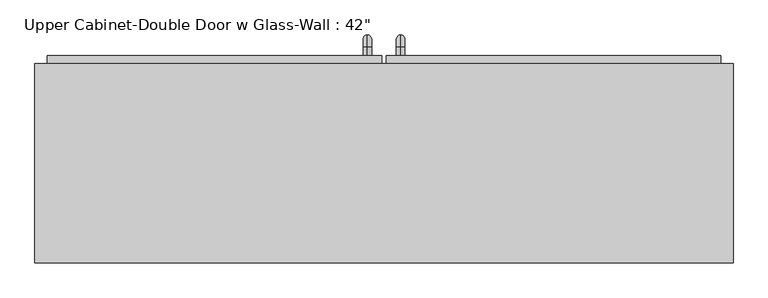
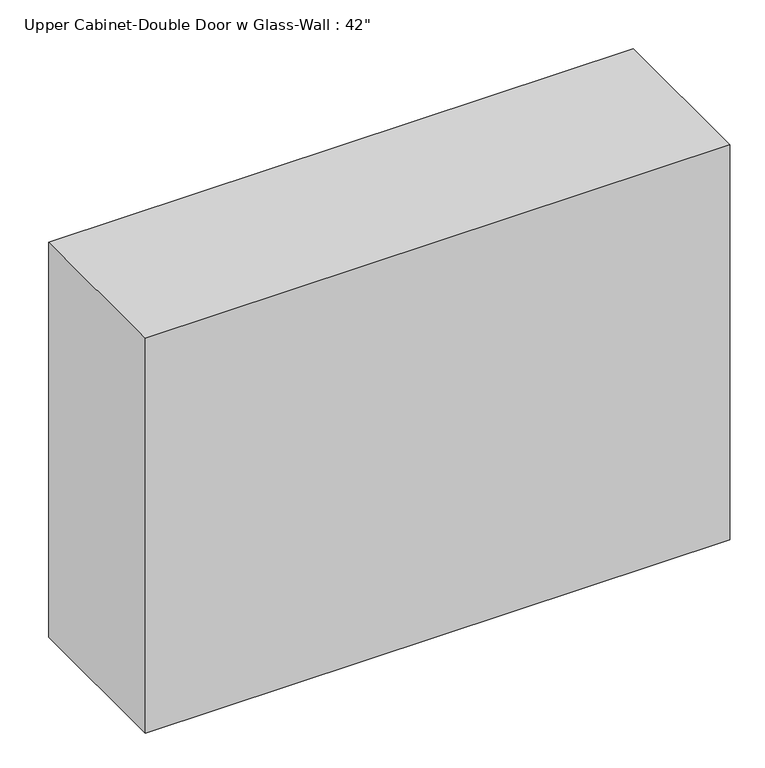
"""IFC4 building model written with IfcOpenShell, lengths in millimetres: furniture geometry."""

from ifc_helpers import new_model, si_unit, point, frame, origin, place, context, project, spatial, polyline, circle_curve, ellipse_curve, trimmed, outline, extrude, faceted_brep, source, transform, mapped, element, save
from ifc_brep_helpers import plane_surface, cylinder_surface, revolved_surface, advanced_brep


def furniture_19fd8281(model_context):
    return source(origin(), model_context, "Body", "SolidModel", [
        extrude(outline(polyline([(2114.55, 32.9461628), (1390.65, 32.9461628), (1390.65, 544.1211628), (2114.55, 544.1211628), (2114.55, 32.9461628)]), holes=[polyline([(1422.4, 64.6961628), (2082.8, 64.6961628), (2082.8, 512.3711628), (1422.4, 512.3711628), (1422.4, 64.6961628)])]), frame((0.0, 400.05, 0.0), z_axis=(0.0, 1.0, 0.0), x_axis=(0.0, 0.0, 1.0)), (0.0, 0.0, 1.0), 31.75),
        extrude(outline(polyline([(1390.65, -484.5788372), (1390.65, 26.5961628), (2114.55, 26.5961628), (2114.55, -484.5788372), (1390.65, -484.5788372)]), holes=[polyline([(2082.8, -5.1538372), (1422.4, -5.1538372), (1422.4, -452.8288372), (2082.8, -452.8288372), (2082.8, -5.1538372)])]), frame((0.0, 400.05, 0.0), z_axis=(0.0, 1.0, 0.0), x_axis=(0.0, 0.0, 1.0)), (0.0, 0.0, 1.0), 31.75),
        extrude(outline(polyline([(64.6961628, 412.75), (512.3711628, 412.75), (512.3711628, 406.4), (64.6961628, 406.4), (64.6961628, 412.75)])), frame((0.0, 0.0, 1422.4), z_axis=(0.0, 0.0, 1.0), x_axis=(1.0, 0.0, 0.0)), (0.0, 0.0, 1.0), 660.4),
        extrude(outline(polyline([(-452.8288372, 412.75), (-5.1538372, 412.75), (-5.1538372, 406.4), (-452.8288372, 406.4), (-452.8288372, 412.75)])), frame((0.0, 0.0, 1422.4), z_axis=(0.0, 0.0, 1.0), x_axis=(1.0, 0.0, 0.0)), (0.0, 0.0, 1.0), 660.4),
        advanced_brep(
        [(4.3711628, 431.8, 1517.65), (4.3711628, 431.8, 1530.35), (4.3711628, 444.5, 1517.65), (4.3711628, 444.5, 1530.35), (4.3711628, 463.55, 1511.3), (4.3711628, 450.85, 1511.3), (4.3711628, 450.85, 1435.1), (4.3711628, 463.55, 1435.1), (4.3711628, 444.5, 1416.05), (4.3711628, 444.5, 1428.75), (4.3711628, 431.8, 1428.75), (4.3711628, 431.8, 1416.05)],
        [
            (0, 1, circle_curve(frame((4.3711628, 431.8, 1524.0), z_axis=(0.0, -1.0, 0.0), x_axis=(0.0, 0.0, 1.0)), 6.35)),
            (1, 0, circle_curve(frame((4.3711628, 431.8, 1524.0), z_axis=(0.0, -1.0, 0.0), x_axis=(0.0, 0.0, 1.0)), 6.35)),
            (0, 2),
            (2, 3, circle_curve(frame((4.3711628, 444.5, 1524.0), z_axis=(0.0, -1.0, 0.0), x_axis=(0.0, 0.0, 1.0)), 6.35)),
            (3, 1),
            (3, 2, circle_curve(frame((4.3711628, 444.5, 1524.0), z_axis=(0.0, -1.0, 0.0), x_axis=(0.0, 0.0, 1.0)), 6.35)),
            (4, 3, circle_curve(frame((4.3711628, 444.5, 1511.3), z_axis=(1.0, 0.0, 0.0), x_axis=(0.0, 0.0, 1.0)), 19.05)),
            (2, 5, circle_curve(frame((4.3711628, 444.5, 1511.3), z_axis=(-1.0, 0.0, 0.0), x_axis=(0.0, 0.0, 1.0)), 6.35)),
            (5, 4, circle_curve(frame((4.3711628, 457.2, 1511.3), z_axis=(0.0, 0.0, 1.0), x_axis=(0.0, 1.0, 0.0)), 6.35)),
            (4, 5, circle_curve(frame((4.3711628, 457.2, 1511.3), z_axis=(0.0, 0.0, 1.0), x_axis=(0.0, 1.0, 0.0)), 6.35)),
            (5, 6),
            (6, 7, circle_curve(frame((4.3711628, 457.2, 1435.1), z_axis=(0.0, 0.0, 1.0), x_axis=(0.0, 1.0, 0.0)), 6.35)),
            (7, 4),
            (7, 6, circle_curve(frame((4.3711628, 457.2, 1435.1), z_axis=(0.0, 0.0, 1.0), x_axis=(0.0, 1.0, 0.0)), 6.35)),
            (8, 7, circle_curve(frame((4.3711628, 444.5, 1435.1), z_axis=(1.0, 0.0, 0.0), x_axis=(0.0, 1.0, 0.0)), 19.05)),
            (6, 9, circle_curve(frame((4.3711628, 444.5, 1435.1), z_axis=(-1.0, 0.0, 0.0), x_axis=(0.0, 1.0, 0.0)), 6.35)),
            (9, 8, circle_curve(frame((4.3711628, 444.5, 1422.4), z_axis=(0.0, 1.0, 0.0), x_axis=(0.0, 0.0, -1.0)), 6.35)),
            (8, 9, circle_curve(frame((4.3711628, 444.5, 1422.4), z_axis=(0.0, 1.0, 0.0), x_axis=(0.0, 0.0, -1.0)), 6.35)),
            (10, 11, circle_curve(frame((4.3711628, 431.8, 1422.4), z_axis=(0.0, -1.0, 0.0), x_axis=(0.0, 0.0, -1.0)), 6.35)),
            (11, 10, circle_curve(frame((4.3711628, 431.8, 1422.4), z_axis=(0.0, -1.0, 0.0), x_axis=(0.0, 0.0, -1.0)), 6.35)),
            (9, 10),
            (11, 8),
        ],
        [
            plane_surface(frame((-1.9788372, 431.8, 1524.0), z_axis=(0.0, -1.0, 0.0), x_axis=(0.0, 0.0, 1.0))),
            cylinder_surface(frame((4.3711628, 431.8, 1524.0), z_axis=(0.0, -1.0, 0.0), x_axis=(0.0, 0.0, 1.0)), 6.35),
            revolved_surface(trimmed(ellipse_curve(frame((4.3711628, 444.5, 1524.0), z_axis=(0.0, -1.0, 0.0), x_axis=(0.0, 0.0, 1.0)), 6.35, 6.35), [point((4.3711628, 444.5, 1517.65))], [point((4.3711628, 444.5, 1530.35))], True, "CARTESIAN"), (4.3711628, 444.5, 1511.3), (-1.0, 0.0, 0.0)),
            revolved_surface(trimmed(ellipse_curve(frame((4.3711628, 444.5, 1524.0), z_axis=(0.0, -1.0, 0.0), x_axis=(0.0, 0.0, 1.0)), 6.35, 6.35), [point((4.3711628, 444.5, 1530.35))], [point((4.3711628, 444.5, 1517.65))], True, "CARTESIAN"), (4.3711628, 444.5, 1511.3), (-1.0, 0.0, 0.0)),
            cylinder_surface(frame((4.3711628, 457.2, 1511.3), z_axis=(0.0, 0.0, 1.0), x_axis=(0.0, 1.0, 0.0)), 6.35),
            revolved_surface(trimmed(ellipse_curve(frame((4.3711628, 457.2, 1435.1), z_axis=(0.0, 0.0, 1.0), x_axis=(0.0, 1.0, 0.0)), 6.35, 6.35), [point((4.3711628, 450.85, 1435.1))], [point((4.3711628, 463.55, 1435.1))], True, "CARTESIAN"), (4.3711628, 444.5, 1435.1), (-1.0, 0.0, 0.0)),
            revolved_surface(trimmed(ellipse_curve(frame((4.3711628, 457.2, 1435.1), z_axis=(0.0, 0.0, 1.0), x_axis=(0.0, 1.0, 0.0)), 6.35, 6.35), [point((4.3711628, 463.55, 1435.1))], [point((4.3711628, 450.85, 1435.1))], True, "CARTESIAN"), (4.3711628, 444.5, 1435.1), (-1.0, 0.0, 0.0)),
            plane_surface(frame((-1.9788372, 431.8, 1422.4), z_axis=(0.0, -1.0, 0.0), x_axis=(0.0, 0.0, -1.0))),
            cylinder_surface(frame((4.3711628, 444.5, 1422.4), z_axis=(0.0, 1.0, 0.0), x_axis=(0.0, 0.0, -1.0)), 6.35),
        ],
        [
            (0, [[1, 2]]),
            (1, [[-1, 3, 4, 5]]),
            (1, [[-2, -5, 6, -3]]),
            (2, [[7, -4, 8, 9]]),
            (3, [[-8, -6, -7, 10]]),
            (4, [[-9, 11, 12, 13]]),
            (4, [[-10, -13, 14, -11]]),
            (5, [[15, -12, 16, 17]]),
            (6, [[-16, -14, -15, 18]]),
            (7, [[19, 20]]),
            (8, [[-17, 21, -20, 22]]),
            (8, [[-18, -22, -19, -21]]),
        ],
    ),
        advanced_brep(
        [(55.1711628, 431.8, 1517.65), (55.1711628, 431.8, 1530.35), (55.1711628, 444.5, 1517.65), (55.1711628, 444.5, 1530.35), (55.1711628, 463.55, 1511.3), (55.1711628, 450.85, 1511.3), (55.1711628, 450.85, 1435.1), (55.1711628, 463.55, 1435.1), (55.1711628, 444.5, 1416.05), (55.1711628, 444.5, 1428.75), (55.1711628, 431.8, 1428.75), (55.1711628, 431.8, 1416.05)],
        [
            (0, 1, circle_curve(frame((55.1711628, 431.8, 1524.0), z_axis=(0.0, -1.0, 0.0), x_axis=(0.0, 0.0, -1.0)), 6.35)),
            (1, 0, circle_curve(frame((55.1711628, 431.8, 1524.0), z_axis=(0.0, -1.0, 0.0), x_axis=(0.0, 0.0, -1.0)), 6.35)),
            (0, 2),
            (2, 3, circle_curve(frame((55.1711628, 444.5, 1524.0), z_axis=(0.0, -1.0, 0.0), x_axis=(0.0, 0.0, -1.0)), 6.35)),
            (3, 1),
            (3, 2, circle_curve(frame((55.1711628, 444.5, 1524.0), z_axis=(0.0, -1.0, 0.0), x_axis=(0.0, 0.0, -1.0)), 6.35)),
            (4, 3, circle_curve(frame((55.1711628, 444.5, 1511.3), z_axis=(1.0, 0.0, 0.0), x_axis=(0.0, 0.0, 1.0)), 19.05)),
            (2, 5, circle_curve(frame((55.1711628, 444.5, 1511.3), z_axis=(-1.0, 0.0, 0.0), x_axis=(0.0, 0.0, 1.0)), 6.35)),
            (5, 4, circle_curve(frame((55.1711628, 457.2, 1511.3), z_axis=(0.0, 0.0, 1.0), x_axis=(0.0, -1.0, 0.0)), 6.35)),
            (4, 5, circle_curve(frame((55.1711628, 457.2, 1511.3), z_axis=(0.0, 0.0, 1.0), x_axis=(0.0, -1.0, 0.0)), 6.35)),
            (5, 6),
            (6, 7, circle_curve(frame((55.1711628, 457.2, 1435.1), z_axis=(0.0, 0.0, 1.0), x_axis=(0.0, -1.0, 0.0)), 6.35)),
            (7, 4),
            (7, 6, circle_curve(frame((55.1711628, 457.2, 1435.1), z_axis=(0.0, 0.0, 1.0), x_axis=(0.0, -1.0, 0.0)), 6.35)),
            (8, 7, circle_curve(frame((55.1711628, 444.5, 1435.1), z_axis=(1.0, 0.0, 0.0), x_axis=(0.0, 1.0, 0.0)), 19.05)),
            (6, 9, circle_curve(frame((55.1711628, 444.5, 1435.1), z_axis=(-1.0, 0.0, 0.0), x_axis=(0.0, 1.0, 0.0)), 6.35)),
            (9, 8, circle_curve(frame((55.1711628, 444.5, 1422.4), z_axis=(0.0, 1.0, 0.0), x_axis=(0.0, 0.0, 1.0)), 6.35)),
            (8, 9, circle_curve(frame((55.1711628, 444.5, 1422.4), z_axis=(0.0, 1.0, 0.0), x_axis=(0.0, 0.0, 1.0)), 6.35)),
            (10, 11, circle_curve(frame((55.1711628, 431.8, 1422.4), z_axis=(0.0, -1.0, 0.0), x_axis=(0.0, 0.0, 1.0)), 6.35)),
            (11, 10, circle_curve(frame((55.1711628, 431.8, 1422.4), z_axis=(0.0, -1.0, 0.0), x_axis=(0.0, 0.0, 1.0)), 6.35)),
            (9, 10),
            (11, 8),
        ],
        [
            plane_surface(frame((48.8211628, 431.8, 1524.0), z_axis=(0.0, -1.0, 0.0), x_axis=(0.0, 0.0, 1.0))),
            cylinder_surface(frame((55.1711628, 431.8, 1524.0), z_axis=(0.0, -1.0, 0.0), x_axis=(0.0, 0.0, -1.0)), 6.35),
            revolved_surface(trimmed(ellipse_curve(frame((55.1711628, 444.5, 1524.0), z_axis=(0.0, -1.0, 0.0), x_axis=(0.0, 0.0, -1.0)), 6.35, 6.35), [point((55.1711628, 444.5, 1517.65))], [point((55.1711628, 444.5, 1530.35))], True, "CARTESIAN"), (55.1711628, 444.5, 1511.3), (-1.0, 0.0, 0.0)),
            revolved_surface(trimmed(ellipse_curve(frame((55.1711628, 444.5, 1524.0), z_axis=(0.0, -1.0, 0.0), x_axis=(0.0, 0.0, -1.0)), 6.35, 6.35), [point((55.1711628, 444.5, 1530.35))], [point((55.1711628, 444.5, 1517.65))], True, "CARTESIAN"), (55.1711628, 444.5, 1511.3), (-1.0, 0.0, 0.0)),
            cylinder_surface(frame((55.1711628, 457.2, 1511.3), z_axis=(0.0, 0.0, 1.0), x_axis=(0.0, -1.0, 0.0)), 6.35),
            revolved_surface(trimmed(ellipse_curve(frame((55.1711628, 457.2, 1435.1), z_axis=(0.0, 0.0, 1.0), x_axis=(0.0, -1.0, 0.0)), 6.35, 6.35), [point((55.1711628, 450.85, 1435.1))], [point((55.1711628, 463.55, 1435.1))], True, "CARTESIAN"), (55.1711628, 444.5, 1435.1), (-1.0, 0.0, 0.0)),
            revolved_surface(trimmed(ellipse_curve(frame((55.1711628, 457.2, 1435.1), z_axis=(0.0, 0.0, 1.0), x_axis=(0.0, -1.0, 0.0)), 6.35, 6.35), [point((55.1711628, 463.55, 1435.1))], [point((55.1711628, 450.85, 1435.1))], True, "CARTESIAN"), (55.1711628, 444.5, 1435.1), (-1.0, 0.0, 0.0)),
            plane_surface(frame((48.8211628, 431.8, 1422.4), z_axis=(0.0, -1.0, 0.0), x_axis=(0.0, 0.0, -1.0))),
            cylinder_surface(frame((55.1711628, 444.5, 1422.4), z_axis=(0.0, 1.0, 0.0), x_axis=(0.0, 0.0, 1.0)), 6.35),
        ],
        [
            (0, [[1, 2]]),
            (1, [[-1, 3, 4, 5]]),
            (1, [[-2, -5, 6, -3]]),
            (2, [[7, -4, 8, 9]]),
            (3, [[-8, -6, -7, 10]]),
            (4, [[-9, 11, 12, 13]]),
            (4, [[-10, -13, 14, -11]]),
            (5, [[15, -12, 16, 17]]),
            (6, [[-16, -14, -15, 18]]),
            (7, [[19, 20]]),
            (8, [[-17, 21, -20, 22]]),
            (8, [[-18, -22, -19, -21]]),
        ],
    ),
        faceted_brep([(-503.6288372, 114.3, 2133.6), (-503.6288372, 114.3, 1371.6), (563.1711628, 114.3, 1371.6), (563.1711628, 114.3, 2133.6), (-503.6288372, 419.1, 2133.6), (563.1711628, 419.1, 2133.6), (563.1711628, 419.1, 1371.6), (-503.6288372, 419.1, 1371.6), (-484.5788372, 419.1, 2114.55), (-484.5788372, 419.1, 1390.65), (544.1211628, 419.1, 1390.65), (544.1211628, 419.1, 2114.55), (544.1211628, 133.35, 2114.55), (-484.5788372, 133.35, 2114.55), (544.1211628, 133.35, 1390.65), (-484.5788372, 133.35, 1390.65)], [[[0, 1, 2, 3]], [[4, 5, 6, 7], [8, 9, 10, 11]], [[1, 0, 4, 7]], [[2, 1, 7, 6]], [[3, 2, 6, 5]], [[0, 3, 5, 4]], [[8, 11, 12, 13]], [[11, 10, 14, 12]], [[10, 9, 15, 14]], [[9, 8, 13, 15]], [[13, 12, 14, 15]]]),
    ])


if __name__ == "__main__":
    model = new_model("IFC4")
    model_context = context("Model", 3, world=origin())
    ifc_project = project(units=[si_unit("LENGTHUNIT", "METRE", prefix="MILLI")], contexts=[model_context])
    site = spatial("IfcSite", under=ifc_project)
    building = spatial("IfcBuilding", under=site)
    placement = place(None, origin())
    furniture_shape = furniture_19fd8281(model_context)
    element("IfcFurniture", 1, ObjectType="Upper Cabinet-Double Door w Glass-Wall : 42\"", at=placement, inside=building, context=model_context, shape_type="MappedRepresentation", body=[
        mapped(furniture_shape, transform((0.0, 0.0, 0.0), x_axis=(1.0, 0.0, 0.0), y_axis=(0.0, 1.0, 0.0), z_axis=(0.0, 0.0, 1.0))),
    ])
    save(model, "model.ifc")

# Revit data of these elements
# Type "Upper Cabinet-Double Door w Glass-Wall : 42\""
#   Assembly Code = "C1030410"
#   Depth = 1' - 0"
#   Height = 2' - 6"
#   Top Of Cabinet = 7' - 0"
#   Width = 3' - 6"
#   Cabinet Material = none
#   Door/Drawer Material = none
#   Handle Material = Cabinets - Handles
#   Panel Material = Glass
#   Default Elevation = 0
# Element 1 (IfcFurniture, "Upper Cabinet-Double Door w Glass-Wall : 42\"")
#   Materials on its faces: "Cabinets", "Cabinets - Handles", "Glass"
# Materials
#   "Cabinets - Handles": colour RGB 57 57 57, transparency 0
#   "Glass": class "Glass", colour RGB 0 128 192, transparency 0.75, Description = "Soda Lime Glass", Cost = 0
#   "Cabinets": colour RGB 249 249 249, transparency 0
